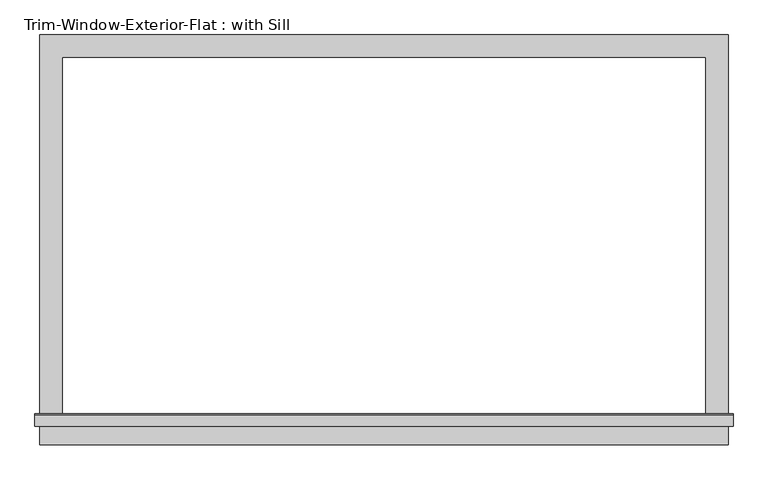
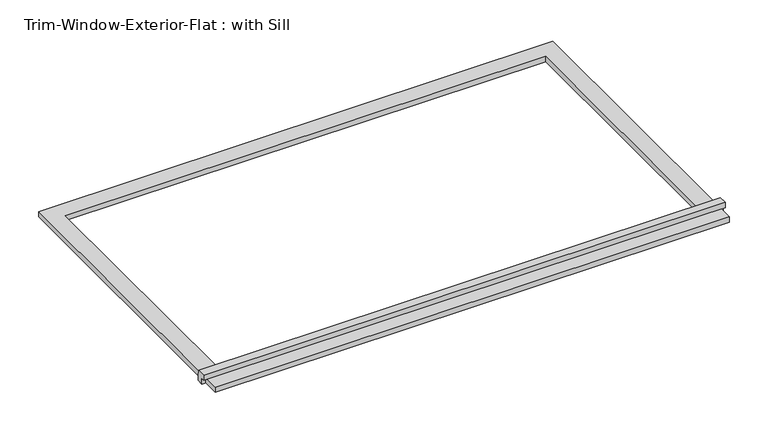
"""IFC4 building model written with IfcOpenShell, lengths in millimetres: proxy geometry, Trim-Window-Exterior-Flat : with Sill."""

from ifc_helpers import new_model, si_unit, frame, origin, origin_with_axes, place, context, project, spatial, polyline, outline, extrude, source, transform, mapped, element, save


def trim_window_exterior_flat_with_sill_c3f87112(model_context):
    return source(origin(), model_context, "Body", "SweptSolid", [
        extrude(outline(polyline([(882.65, -936.5823709), (882.65, -993.7323709), (-882.65, -993.7323709), (-882.65, -936.5823709), (882.65, -936.5823709)])), origin_with_axes(), (0.0, 0.0, 1.0), 19.05),
        extrude(outline(polyline([(-946.15, 38.1), (-916.8580645, 38.1), (-914.4, 19.05), (-914.4, 0.0), (-936.5823709, 0.0), (-936.5823709, 19.05), (-946.15, 19.05), (-946.15, 38.1)])), frame((-895.35, 0.0, 0.0), z_axis=(1.0, 0.0, 0.0), x_axis=(0.0, 1.0, 0.0)), (0.0, 0.0, 1.0), 1790.7),
        extrude(outline(polyline([(-882.65, 57.15), (882.65, 57.15), (882.65, -914.4), (825.5, -914.4), (825.5, 0.0), (-825.5, 0.0), (-825.5, -914.4), (-882.65, -914.4), (-882.65, 57.15)])), origin_with_axes(), (0.0, 0.0, 1.0), 19.05),
    ])


if __name__ == "__main__":
    model = new_model("IFC4")
    model_context = context("Model", 3, world=origin())
    ifc_project = project(units=[si_unit("LENGTHUNIT", "METRE", prefix="MILLI")], contexts=[model_context])
    site = spatial("IfcSite", under=ifc_project)
    building = spatial("IfcBuilding", under=site)
    placement = place(None, origin())
    trim_window_exterior_flat_with_sill_shape = trim_window_exterior_flat_with_sill_c3f87112(model_context)
    element("IfcBuildingElementProxy", 1, Name="Trim-Window-Exterior-Flat : with Sill", ObjectType="Trim-Window-Exterior-Flat : with Sill", at=placement, inside=building, context=model_context, shape_type="MappedRepresentation", body=[
        mapped(trim_window_exterior_flat_with_sill_shape, transform((0.0, 0.0, 0.0), x_axis=(1.0, 0.0, 0.0), y_axis=(0.0, 1.0, 0.0), z_axis=(0.0, 0.0, 1.0))),
    ])
    save(model, "model.ifc")

# Revit data of these elements
# Type "Trim-Window-Exterior-Flat : with Sill"
#   Trim Width = 0' - 2 1/4"
#   Trim Thickness_Picture Frame = 0' - 1 1/4"
#   Trim Thickness_with Sill = 0' - 0 3/4"
#   Sill Thickness = 0' - 1 1/4"
#   Opening Width [instance default] = 2' - 0"
#   Opening Height [instance default] = 3' - 0"
#   Default Elevation = 4' - 0"
#   Sill = yes
#   Picture Frame = no
#   Trim Material [instance default] = none
# Element 1 (IfcBuildingElementProxy, "Trim-Window-Exterior-Flat : with Sill")
#   Opening Width = 5' - 5"
#   Trim Material = Clad - White
#   Materials on its faces: "Clad - White"
# Materials
#   "Clad - White": class "Wood", colour RGB 242 242 238, transparency 0, Cost = 0
